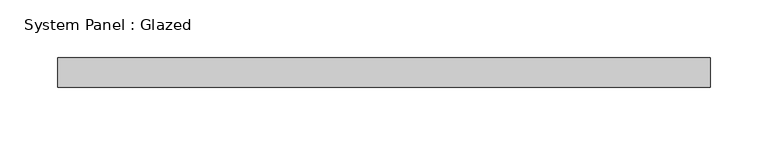
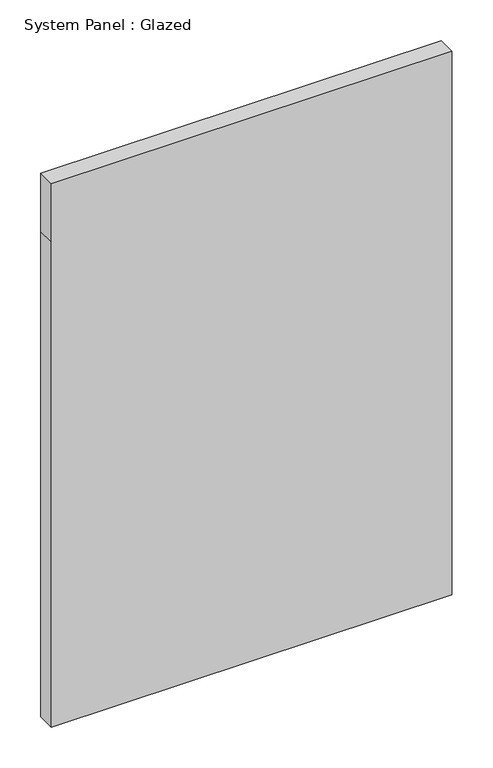
"""IFC4 building model written with IfcOpenShell, lengths in millimetres: plate geometry, System Panel : Glazed."""

from ifc_helpers import new_model, si_unit, frame, origin, place, context, project, spatial, polyline, outline, extrude, source, transform, mapped, element, save


def system_panel_glazed_f743f071(model_context):
    return source(origin(), model_context, "Body", "SweptSolid", [
        extrude(outline(polyline([(0.0, -282.575), (0.0, 282.575), (723.9, 282.575), (810.6833333, 282.575), (810.6833333, -282.575), (723.9, -282.575), (0.0, -282.575)])), frame((0.0, 19.05, 0.0), z_axis=(0.0, 1.0, 0.0), x_axis=(0.0, 0.0, 1.0)), (0.0, 0.0, 1.0), 25.4),
    ])


if __name__ == "__main__":
    model = new_model("IFC4")
    model_context = context("Model", 3, world=origin())
    ifc_project = project(units=[si_unit("LENGTHUNIT", "METRE", prefix="MILLI")], contexts=[model_context])
    site = spatial("IfcSite", under=ifc_project)
    building = spatial("IfcBuilding", under=site)
    placement = place(None, origin())
    system_panel_glazed_shape = system_panel_glazed_f743f071(model_context)
    element("IfcPlate", 1, ObjectType="System Panel : Glazed", at=placement, inside=building, context=model_context, shape_type="MappedRepresentation", body=[
        mapped(system_panel_glazed_shape, transform((0.0, 0.0, 0.0), x_axis=(1.0, 0.0, 0.0), y_axis=(0.0, 1.0, 0.0), z_axis=(0.0, 0.0, 1.0))),
    ])
    save(model, "model.ifc")

# Revit data of these elements
# Type "System Panel : Glazed"
#   Construction Type Id = "GSP4R"
#   Analytic Construction = "1/8 in Pilkington single glazing"
#   Visual Light Transmittance = 0.9
#   Solar Heat Gain Coefficient = 0.86
#   Heat Transfer Coefficient (U) = 1.18115 BTU/(h·ft²·°F)
#   Define Thermal Properties by = 1
# Element 1 (IfcPlate, "System Panel : Glazed")
#   Materials on its faces: "Glass"
# Materials
#   "Glass": class "Glass", colour RGB 0 128 192, transparency 0.75, Description = "Soda Lime Glass", Cost = 0
